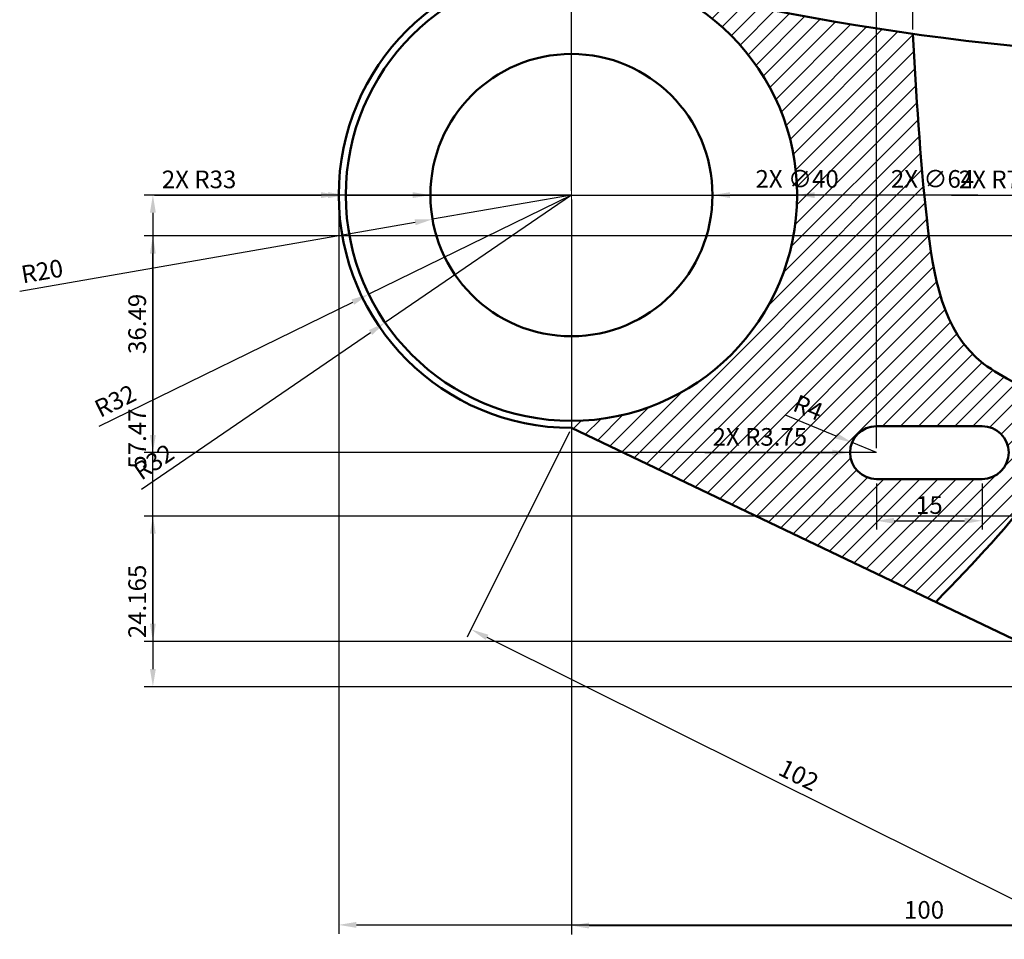
# Model space of a CAD drawing. Units: millimetres. Extents: x 1605 to 2079, y 1280 to 1879.
# Tile 2 of 7: x 1605 to 1745, y 1384 to 1514. Entities that reach past the tile are written whole.
import ezdxf

# ---------------------------------------------------------------- set-up
doc = ezdxf.new("R2010")
doc.units = ezdxf.units.MM
doc.linetypes.add('CENTER2', pattern=[28.574999999999996, 19.05, -3.174999999999999, 3.174999999999999, -3.174999999999999])
for name, color, linetype, lineweight in [('M-CNTR', 1, 'CENTER2', 18), ('M-DIMS', 2, 'Continuous', 25), ('M-HATC', 8, 'Continuous', 18), ('M-OUTL', 7, 'Continuous', 50)]:
    doc.layers.add(name, color=color, linetype=linetype, lineweight=lineweight)
doc.styles.get("Standard").update_dxf_attribs({"font": 'arial.ttf'})
doc.dimstyles.new('ISO-25', dxfattribs={"dimtxt": 2.5, "dimasz": 2.5, "dimexe": 1.25, "dimexo": 0.625, "dimtad": 1, "dimdec": 0, "dimtxsty": 'Standard', "dimcen": 2.5, "dimadec": 0, "dimazin": 0, "dimtfac": 1, "dimtdec": 0, "dimtmove": 0, "dimatfit": 3, "dimfxl": 1, "dimarcsym": 0})

# ---------------------------------------------------------------- blocks, each defined once
blk = doc.blocks.new('*U2')
at = {"layer": 'M-CNTR', "color": 0, "transparency": 16777216}
for p, q in [((0, 6.4), (0, 35.5)), ((-35.5, 0), (-6.399999999999998, 0)), ((6.4, 0), (35.5, 0)), ((0, -35.5), (0, -6.399999999999998))]:
    blk.add_line(p, q, dxfattribs=at)
at = {"layer": 'M-CNTR', "color": 0, "linetype": 'Continuous', "transparency": 16777216}
for p, q in [((0, -3.2), (0, 3.2)), ((-3.2, 0), (3.2, 0))]:
    blk.add_line(p, q, dxfattribs=at)
blk = doc.blocks.new('*D12')
at = {"layer": 'Defpoints', "color": 0, "transparency": 16777216}
for p in [(1650.415855978972, 1488.98060105796), (1916.415855978972, 1488.98060105796), (1916.415855978972, 1385.555788157088)]:
    blk.add_point(p, dxfattribs=at)
at = {"layer": 'M-DIMS', "color": 0, "lineweight": -2, "transparency": 16777216}
for p, q in [((1650.415855978972, 1488.35560105796), (1650.415855978972, 1384.305788157088)), ((1916.415855978972, 1488.35560105796), (1916.415855978972, 1384.305788157088)), ((1652.915855978972, 1385.555788157088), (1913.915855978972, 1385.555788157088))]:
    blk.add_line(p, q, dxfattribs=at)
at = {"layer": 'M-DIMS', "color": 0, "transparency": 16777216}
for points in [[(1652.915855978972, 1385.972454823755), (1652.915855978972, 1385.139121490422), (1650.415855978972, 1385.555788157088)], [(1913.915855978972, 1385.972454823755), (1913.915855978972, 1385.139121490422), (1916.415855978972, 1385.555788157088)]]:
    blk.add_solid(points, dxfattribs=at)
at = {"layer": 'M-DIMS', "color": 0, "transparency": 16777216, "insert": (1783.415855978972, 1387.457220626393), "char_height": 2.5, "attachment_point": 5}
blk.add_mtext('266', dxfattribs=at)
blk = doc.blocks.new('*D14')
at = {"layer": 'Defpoints', "color": 0, "transparency": 16777216}
for p in [(1683.415855978973, 1488.98060105796), (1654.670127227685, 1474.920619601452)]:
    blk.add_point(p, dxfattribs=at)
at = {"layer": 'M-DIMS', "color": 0, "lineweight": -2, "transparency": 16777216}
for p, q in [((1683.415855978973, 1488.98060105796), (1654.670127227685, 1474.920619601452)), ((1616.470490142547, 1456.236585054639), (1652.42436716899, 1473.822183550162))]:
    blk.add_line(p, q, dxfattribs=at)
at = {"layer": 'M-DIMS', "color": 0, "transparency": 16777216}
blk.add_solid([(1652.241294493775, 1474.196476893278), (1652.607439844205, 1473.447890207046), (1654.670127227685, 1474.920619601452)], dxfattribs=at)
at = {"layer": 'M-DIMS', "color": 0, "transparency": 16777216, "insert": (1618.867741976558, 1459.526758746126), "char_height": 2.5, "attachment_point": 5, "rotation": 26.063973519573043}
blk.add_mtext('R32', dxfattribs=at)
blk = doc.blocks.new('*D15')
at = {"layer": 'Defpoints', "color": 0, "transparency": 16777216}
for p in [(1683.415855978971, 1488.98060105796), (1656.997927559478, 1470.92255415298)]:
    blk.add_point(p, dxfattribs=at)
at = {"layer": 'M-DIMS', "color": 0, "lineweight": -2, "transparency": 16777216}
for p, q in [((1683.415855978971, 1488.98060105796), (1656.997927559478, 1470.92255415298)), ((1622.466120198724, 1447.318243204279), (1654.934026901705, 1469.511769238528))]:
    blk.add_line(p, q, dxfattribs=at)
at = {"layer": 'M-DIMS', "color": 0, "transparency": 16777216}
blk.add_solid([(1654.69889608263, 1469.85575268149), (1655.16915772078, 1469.167785795566), (1656.997927559478, 1470.92255415298)], dxfattribs=at)
at = {"layer": 'M-DIMS', "color": 0, "transparency": 16777216, "insert": (1624.363890844126, 1450.919704831629), "char_height": 2.5, "attachment_point": 5, "rotation": 34.354665422321524}
blk.add_mtext('R32', dxfattribs=at)
blk = doc.blocks.new('*D16')
at = {"layer": 'Defpoints', "color": 0, "transparency": 16777216}
for p in [(1683.415855978971, 1488.980601057959), (1663.711259292998, 1485.555857353229)]:
    blk.add_point(p, dxfattribs=at)
at = {"layer": 'M-DIMS', "color": 0, "lineweight": -2, "transparency": 16777216}
for p, q in [((1683.415855978971, 1488.980601057959), (1663.711259292998, 1485.555857353229)), ((1605.180206259197, 1475.382908441698), (1661.248184707251, 1485.127764390138))]:
    blk.add_line(p, q, dxfattribs=at)
at = {"layer": 'M-DIMS', "color": 0, "transparency": 16777216}
blk.add_solid([(1661.176835880069, 1485.538276821096), (1661.319533534433, 1484.71725195918), (1663.711259292998, 1485.555857353229)], dxfattribs=at)
at = {"layer": 'M-DIMS', "color": 0, "transparency": 16777216, "insert": (1608.408931110697, 1477.874012688988), "char_height": 2.5, "attachment_point": 5, "rotation": 9.859759404973948}
blk.add_mtext('R20', dxfattribs=at)
blk = doc.blocks.new('*D24')
at = {"layer": 'Defpoints', "color": 0, "transparency": 16777216}
for p in [(1683.415855978972, 1455.980601057961), (1774.34023088235, 1410.708833274267), (1760.124148162526, 1382.157077993787)]:
    blk.add_point(p, dxfattribs=at)
at = {"layer": 'M-DIMS', "color": 0, "lineweight": -2, "transparency": 16777216}
for p, q in [((1683.1372852421, 1455.421116165798), (1668.642631785403, 1426.309875993155)), ((1671.437712827799, 1426.314562829992), (1757.886208593874, 1383.271360941276)), ((1774.061660145477, 1410.149348382104), (1759.567006688781, 1381.038108209462))]:
    blk.add_line(p, q, dxfattribs=at)
at = {"layer": 'M-DIMS', "color": 0, "transparency": 16777216}
for points in [[(1671.623426652381, 1426.6875527581), (1671.251999003217, 1425.941572901883), (1669.199773259148, 1427.42884577748)], [(1758.071922418456, 1383.644350869385), (1757.700494769293, 1382.898371013168), (1760.124148162526, 1382.157077993787)]]:
    blk.add_solid(points, dxfattribs=at)
at = {"layer": 'M-DIMS', "color": 0, "transparency": 16777216, "insert": (1715.509454221376, 1406.495078269704), "char_height": 2.5, "attachment_point": 5, "rotation": 333.5310232172807}
blk.add_mtext('102', dxfattribs=at)
blk = doc.blocks.new('*D26')
at = {"layer": 'Defpoints', "color": 0, "transparency": 16777216}
for p in [(1726.66629323774, 1448.737829432783), (1741.66629323774, 1448.737829432783), (1741.66629323774, 1442.830488730683)]:
    blk.add_point(p, dxfattribs=at)
at = {"layer": 'M-DIMS', "color": 0, "lineweight": -2, "transparency": 16777216}
for p, q in [((1726.66629323774, 1448.112829432783), (1726.66629323774, 1441.580488730683)), ((1741.66629323774, 1448.112829432783), (1741.66629323774, 1441.580488730683)), ((1729.16629323774, 1442.830488730683), (1739.16629323774, 1442.830488730683))]:
    blk.add_line(p, q, dxfattribs=at)
at = {"layer": 'M-DIMS', "color": 0, "transparency": 16777216}
for points in [[(1729.16629323774, 1443.24715539735), (1729.16629323774, 1442.413822064016), (1726.66629323774, 1442.830488730683)], [(1739.16629323774, 1443.24715539735), (1739.16629323774, 1442.413822064016), (1741.66629323774, 1442.830488730683)]]:
    blk.add_solid(points, dxfattribs=at)
at = {"layer": 'M-DIMS', "color": 0, "transparency": 16777216, "insert": (1734.16629323774, 1444.731921199987), "char_height": 2.5, "attachment_point": 5}
blk.add_mtext('15', dxfattribs=at)
blk = doc.blocks.new('*D27')
at = {"layer": 'Defpoints', "color": 0, "transparency": 16777216}
for p in [(1723.201111272499, 1453.921361416299), (1726.666293237741, 1452.487829432783)]:
    blk.add_point(p, dxfattribs=at)
at = {"layer": 'M-DIMS', "color": 0, "lineweight": -2, "transparency": 16777216}
for p, q in [((1713.710073993439, 1457.84776575314), (1720.890989962337, 1454.877049405309)), ((1726.666293237741, 1452.487829432783), (1723.201111272499, 1453.921361416299))]:
    blk.add_line(p, q, dxfattribs=at)
at = {"layer": 'M-DIMS', "color": 0, "transparency": 16777216}
blk.add_solid([(1721.050271293839, 1455.262069623669), (1720.731708630835, 1454.492029186949), (1723.201111272499, 1453.921361416299)], dxfattribs=at)
at = {"layer": 'M-DIMS', "color": 0, "transparency": 16777216, "insert": (1716.862237314565, 1458.57284255635), "char_height": 2.5, "attachment_point": 5, "rotation": 337.52531510139886}
blk.add_mtext('R4', dxfattribs=at)
blk = doc.blocks.new('*D41')
at = {"layer": 'Defpoints', "color": 0, "transparency": 16777216}
for p in [(1763.415856000001, 1443.479022), (1624.065856000002, 1419.31445), (1783.415856000001, 1419.31445)]:
    blk.add_point(p, dxfattribs=at)
at = {"layer": 'M-DIMS', "color": 0, "lineweight": -2, "transparency": 16777216}
for p, q in [((1762.790856000001, 1443.479022), (1622.815856000002, 1443.479022)), ((1624.065856000002, 1440.979022), (1624.065856000002, 1421.81445)), ((1782.790856000001, 1419.31445), (1622.815856000002, 1419.31445))]:
    blk.add_line(p, q, dxfattribs=at)
at = {"layer": 'M-DIMS', "color": 0, "transparency": 16777216}
for points in [[(1623.649189333335, 1440.979022), (1624.482522666668, 1440.979022), (1624.065856000002, 1443.479022)], [(1623.649189333335, 1421.81445), (1624.482522666668, 1421.81445), (1624.065856000002, 1419.31445)]]:
    blk.add_solid(points, dxfattribs=at)
at = {"layer": 'M-DIMS', "color": 0, "transparency": 16777216, "insert": (1622.164423530697, 1431.396736), "char_height": 2.5, "attachment_point": 5, "rotation": 90}
blk.add_mtext('24.165', dxfattribs=at)
blk = doc.blocks.new('*D42')
at = {"layer": 'Defpoints', "color": 0, "transparency": 16777216}
for p in [(1683.415856, 1488.980601), (1783.415856, 1443.479022), (1783.415856, 1385.46445)]:
    blk.add_point(p, dxfattribs=at)
at = {"layer": 'M-DIMS', "color": 0, "lineweight": -2, "transparency": 16777216}
for p, q in [((1683.415856, 1488.355601), (1683.415856, 1384.21445)), ((1783.415856, 1442.854022), (1783.415856, 1384.21445)), ((1685.915856, 1385.46445), (1780.915856, 1385.46445))]:
    blk.add_line(p, q, dxfattribs=at)
at = {"layer": 'M-DIMS', "color": 0, "transparency": 16777216}
for points in [[(1685.915856, 1385.881116666667), (1685.915856, 1385.047783333333), (1683.415856, 1385.46445)], [(1780.915856, 1385.881116666667), (1780.915856, 1385.047783333333), (1783.415856, 1385.46445)]]:
    blk.add_solid(points, dxfattribs=at)
at = {"layer": 'M-DIMS', "color": 0, "transparency": 16777216, "insert": (1733.415856, 1387.365882469304), "char_height": 2.5, "attachment_point": 5}
blk.add_mtext('100', dxfattribs=at)
blk = doc.blocks.new('*D45')
at = {"layer": 'Defpoints', "color": 0, "transparency": 16777216}
for p in [(1763.415856, 1548.330601), (1683.415856, 1488.980601), (1763.415856, 1488.980601)]:
    blk.add_point(p, dxfattribs=at)
at = {"layer": 'M-DIMS', "color": 0, "lineweight": -2, "transparency": 16777216}
for p, q in [((1683.415856, 1489.605601), (1683.415856, 1549.580601)), ((1685.915856, 1548.330601), (1760.915856, 1548.330601)), ((1763.415856, 1489.605601), (1763.415856, 1549.580601))]:
    blk.add_line(p, q, dxfattribs=at)
at = {"layer": 'M-DIMS', "color": 0, "transparency": 16777216}
for points in [[(1685.915856, 1548.747267666666), (1685.915856, 1547.913934333333), (1683.415856, 1548.330601)], [(1760.915856, 1548.747267666666), (1760.915856, 1547.913934333333), (1763.415856, 1548.330601)]]:
    blk.add_solid(points, dxfattribs=at)
at = {"layer": 'M-DIMS', "color": 0, "transparency": 16777216, "insert": (1723.415856, 1550.232033469304), "char_height": 2.5, "attachment_point": 5}
blk.add_mtext('80', dxfattribs=at)
blk = doc.blocks.new('*D47')
at = {"layer": 'Defpoints', "color": 0, "transparency": 16777216}
for p in [(1726.666293, 1548.330601), (1683.415856, 1488.980601), (1726.666293, 1452.487829)]:
    blk.add_point(p, dxfattribs=at)
at = {"layer": 'M-DIMS', "color": 0, "lineweight": -2, "transparency": 16777216}
for p, q in [((1683.415856, 1489.605601), (1683.415856, 1549.580601)), ((1685.915856, 1548.330601), (1724.166293, 1548.330601)), ((1726.666293, 1453.112829), (1726.666293, 1549.580601))]:
    blk.add_line(p, q, dxfattribs=at)
at = {"layer": 'M-DIMS', "color": 0, "transparency": 16777216}
for points in [[(1685.915856, 1548.747267666666), (1685.915856, 1547.913934333333), (1683.415856, 1548.330601)], [(1724.166293, 1548.747267666666), (1724.166293, 1547.913934333333), (1726.666293, 1548.330601)]]:
    blk.add_solid(points, dxfattribs=at)
at = {"layer": 'M-DIMS', "color": 0, "transparency": 16777216, "insert": (1705.0410745, 1550.232886129604), "char_height": 2.5, "attachment_point": 5}
blk.add_mtext('43.25', dxfattribs=at)
blk = doc.blocks.new('*D48')
at = {"layer": 'Defpoints', "color": 0, "transparency": 16777216}
for p in [(1683.415856000001, 1488.980601), (1624.065856000002, 1452.487829), (1726.666293000001, 1452.487829)]:
    blk.add_point(p, dxfattribs=at)
at = {"layer": 'M-DIMS', "color": 0, "lineweight": -2, "transparency": 16777216}
for p, q in [((1682.790856000001, 1488.980601), (1622.815856000002, 1488.980601)), ((1624.065856000002, 1486.480601), (1624.065856000002, 1454.987829)), ((1726.041293000001, 1452.487829), (1622.815856000002, 1452.487829))]:
    blk.add_line(p, q, dxfattribs=at)
at = {"layer": 'M-DIMS', "color": 0, "transparency": 16777216}
for points in [[(1623.649189333335, 1486.480601), (1624.482522666668, 1486.480601), (1624.065856000002, 1488.980601)], [(1623.649189333335, 1454.987829), (1624.482522666668, 1454.987829), (1624.065856000002, 1452.487829)]]:
    blk.add_solid(points, dxfattribs=at)
at = {"layer": 'M-DIMS', "color": 0, "transparency": 16777216, "insert": (1622.163570870397, 1470.734215), "char_height": 2.5, "attachment_point": 5, "rotation": 90}
blk.add_mtext('36.49', dxfattribs=at)
blk = doc.blocks.new('*D49')
at = {"layer": 'Defpoints', "color": 0, "transparency": 16777216}
for p in [(1731.842463, 1548.330601), (1731.842463, 1511.839336), (1683.415856, 1488.980601)]:
    blk.add_point(p, dxfattribs=at)
at = {"layer": 'M-DIMS', "color": 0, "lineweight": -2, "transparency": 16777216}
for p, q in [((1683.415856, 1489.605601), (1683.415856, 1549.580601)), ((1685.915856, 1548.330601), (1729.342463, 1548.330601)), ((1731.842463, 1512.464336), (1731.842463, 1549.580601))]:
    blk.add_line(p, q, dxfattribs=at)
at = {"layer": 'M-DIMS', "color": 0, "transparency": 16777216}
for points in [[(1685.915856, 1548.747267666666), (1685.915856, 1547.913934333333), (1683.415856, 1548.330601)], [(1729.342463, 1548.747267666666), (1729.342463, 1547.913934333333), (1731.842463, 1548.330601)]]:
    blk.add_solid(points, dxfattribs=at)
at = {"layer": 'M-DIMS', "color": 0, "transparency": 16777216, "insert": (1707.6291595, 1550.232886129604), "char_height": 2.5, "attachment_point": 5}
blk.add_mtext('48.43', dxfattribs=at)
blk = doc.blocks.new('*D51')
at = {"layer": 'Defpoints', "color": 0, "transparency": 16777216}
for p in [(1624.065856000002, 1483.204576), (1984.756367000001, 1483.204576), (1947.568769000001, 1425.734399)]:
    blk.add_point(p, dxfattribs=at)
at = {"layer": 'M-DIMS', "color": 0, "lineweight": -2, "transparency": 16777216}
for p, q in [((1984.131367000001, 1483.204576), (1622.815856000002, 1483.204576)), ((1624.065856000002, 1428.234399), (1624.065856000002, 1480.704576000001)), ((1946.943769000001, 1425.734399), (1622.815856000002, 1425.734399))]:
    blk.add_line(p, q, dxfattribs=at)
at = {"layer": 'M-DIMS', "color": 0, "transparency": 16777216}
for points in [[(1623.649189333335, 1480.704576000001), (1624.482522666668, 1480.704576000001), (1624.065856000002, 1483.204576)], [(1623.649189333335, 1428.234399), (1624.482522666668, 1428.234399), (1624.065856000002, 1425.734399)]]:
    blk.add_solid(points, dxfattribs=at)
at = {"layer": 'M-DIMS', "color": 0, "transparency": 16777216, "insert": (1622.169539492498, 1454.4694875), "char_height": 2.5, "attachment_point": 5, "rotation": 90}
blk.add_mtext('57.47', dxfattribs=at)
blk = doc.blocks.new('*D61')
at = {"layer": 'Defpoints', "color": 0, "transparency": 16777216}
for p in [(1650.415856, 1488.981), (1683.415856, 1488.980601)]:
    blk.add_point(p, dxfattribs=at)
at = {"layer": 'M-DIMS', "color": 0, "lineweight": -2, "transparency": 16777216}
for p, q in [((1624.296790517598, 1488.981315803246), (1647.915856000183, 1488.981030227273)), ((1683.415856, 1488.980601), (1650.415856, 1488.981))]:
    blk.add_line(p, q, dxfattribs=at)
at = {"layer": 'M-DIMS', "color": 0, "transparency": 16777216}
blk.add_solid([(1647.915861038061, 1489.397696893909), (1647.915850962304, 1488.564363560636), (1650.415856, 1488.981)], dxfattribs=at)
at = {"layer": 'M-DIMS', "color": 0, "transparency": 16777216, "insert": (1630.615879001804, 1490.883524529465), "char_height": 2.5, "attachment_point": 5, "rotation": 359.9993072419386}
blk.add_mtext('2X R33', dxfattribs=at)
blk = doc.blocks.new('*D62')
at = {"layer": 'Defpoints', "color": 0, "transparency": 16777216}
for p in [(1651.415856, 1488.980202), (1715.415856, 1488.981)]:
    blk.add_point(p, dxfattribs=at)
at = {"layer": 'M-DIMS', "color": 0, "lineweight": -2, "transparency": 16777216}
for p, q in [((1648.915856000195, 1488.980170828124), (1646.415856000389, 1488.980139656249)), ((1651.415856, 1488.980202), (1715.415856, 1488.981)), ((1741.027008794735, 1488.981319339061), (1717.915855999805, 1488.981031171875))]:
    blk.add_line(p, q, dxfattribs=at)
at = {"layer": 'M-DIMS', "color": 0, "transparency": 16777216}
for points in [[(1648.915850804882, 1489.396837494759), (1648.915861195507, 1488.56350416149), (1651.415856, 1488.980202)], [(1717.915850804493, 1489.397697838509), (1717.915861195118, 1488.564364505241), (1715.415856, 1488.981)]]:
    blk.add_solid(points, dxfattribs=at)
at = {"layer": 'M-DIMS', "color": 0, "transparency": 16777216, "insert": (1734.61583141823, 1490.952590013762), "char_height": 2.5, "attachment_point": 5, "rotation": 0.0007144067509826848}
blk.add_mtext('2X ∅64', dxfattribs=at)
blk = doc.blocks.new('*D63')
at = {"layer": 'Defpoints', "color": 0, "transparency": 16777216}
for p in [(1663.415856000001, 1488.980202), (1703.415856, 1488.981)]:
    blk.add_point(p, dxfattribs=at)
at = {"layer": 'M-DIMS', "color": 0, "lineweight": -2, "transparency": 16777216}
for p, q in [((1660.915856000498, 1488.980152125), (1658.415856000996, 1488.98010225)), ((1663.415856000001, 1488.980202), (1703.415856, 1488.981)), ((1721.827861453362, 1488.981367319509), (1705.915855999502, 1488.981049875))]:
    blk.add_line(p, q, dxfattribs=at)
at = {"layer": 'M-DIMS', "color": 0, "transparency": 16777216}
for points in [[(1660.915847687998, 1489.396818791584), (1660.915864312998, 1488.563485458416), (1663.415856000001, 1488.980202)], [(1705.915847687002, 1489.397716541584), (1705.915864312003, 1488.564383208416), (1703.415856, 1488.981)]]:
    blk.add_solid(points, dxfattribs=at)
at = {"layer": 'M-DIMS', "color": 0, "transparency": 16777216, "insert": (1715.415816669167, 1490.952590013523), "char_height": 2.5, "attachment_point": 5, "rotation": 0.001143050800851883}
blk.add_mtext('2X ∅40', dxfattribs=at)
blk = doc.blocks.new('*D68')
at = {"layer": 'Defpoints', "color": 0, "transparency": 16777216}
for p in [(1755.915856, 1488.981), (1763.415855999999, 1488.980601)]:
    blk.add_point(p, dxfattribs=at)
at = {"layer": 'M-DIMS', "color": 0, "lineweight": -2, "transparency": 16777216}
for p, q in [((1737.288639109579, 1488.981990967938), (1753.415856003538, 1488.981133)), ((1763.415855999999, 1488.980601), (1755.915856, 1488.981))]:
    blk.add_line(p, q, dxfattribs=at)
at = {"layer": 'M-DIMS', "color": 0, "transparency": 16777216}
blk.add_solid([(1753.415878170204, 1489.397799666077), (1753.415833836871, 1488.564466333922), (1755.915856, 1488.981)], dxfattribs=at)
at = {"layer": 'M-DIMS', "color": 0, "transparency": 16777216, "insert": (1744.102348714535, 1490.883060950582), "char_height": 2.5, "attachment_point": 5, "rotation": 359.99695186453266}
blk.add_mtext('2X R7.5', dxfattribs=at)
blk = doc.blocks.new('*D69')
at = {"layer": 'Defpoints', "color": 0, "transparency": 16777216}
for p in [(1722.916293, 1452.488), (1726.666293, 1452.487829)]:
    blk.add_point(p, dxfattribs=at)
at = {"layer": 'M-DIMS', "color": 0, "lineweight": -2, "transparency": 16777216}
for p, q in [((1702.346715940895, 1452.488937972713), (1720.416293002599, 1452.488114)), ((1726.666293, 1452.487829), (1722.916293, 1452.488))]:
    blk.add_line(p, q, dxfattribs=at)
at = {"layer": 'M-DIMS', "color": 0, "transparency": 16777216}
blk.add_solid([(1720.416312002599, 1452.904780666233), (1720.416274002599, 1452.071447333766), (1722.916293, 1452.488)], dxfattribs=at)
at = {"layer": 'M-DIMS', "color": 0, "transparency": 16777216, "insert": (1710.131591217248, 1454.390868113983), "char_height": 2.5, "attachment_point": 5, "rotation": 359.9973873124574}
blk.add_mtext('2X R3.75', dxfattribs=at)

msp = doc.modelspace()

# ---------------------------------------------------------------- hatches: boundary and pattern name
at = {"layer": 'M-HATC'}
h = msp.add_hatch(dxfattribs=at)
h.set_pattern_fill('ANSI31', color=256, scale=0.5700000000000001)
h.set_pattern_definition([(45, (0, 0), (-1.279686497252354, 1.279686497252354), [])])
edge = h.paths.add_edge_path()
edge.add_spline(control_points=[(1735.07459974606, 1431.314795075923), (1745.983278041014, 1442.572726331581), (1760.24984788448, 1457.296055612093), (1736.483989804082, 1465.949384402775), (1733.184296285201, 1487.573131299177), (1732.318614147286, 1503.228440483471), (1731.842462696298, 1511.83933570387)], knot_values=[0, 0, 0, 0, 32.3106591245444, 42.25647348148218, 64.0151754338639, 90.61240603446909, 90.61240603446909, 90.61240603446909, 90.61240603446909], degree=3, periodic=0)
edge.add_arc((1783.415855978972, 1878.806874192082), 370.5738647001252, 256.0328658121666, 262.00008128327465, ccw=False)
edge.add_arc((1683.415855978972, 1488.98060105796), 32, 0, 70.73817384477002, ccw=False)
edge.add_arc((1683.415855978972, 1488.98060105796), 32, -90, 0, ccw=False)
edge.add_line((1683.415855978972, 1456.98060105796), (1683.415855978972, 1455.98060105796))
edge.add_line((1683.415855978972, 1455.98060105796), (1735.07459974606, 1431.314795075923))
h.paths.add_polyline_path([(1726.66629323774, 1456.237829432783), (1741.66629323774, 1456.237829432783, -1), (1741.66629323774, 1448.737829432783), (1726.66629323774, 1448.737829432783, -1)], flags=16)
h.paths.add_polyline_path([(1731.47870797171, 1442.133012605171), (1736.613428299132, 1442.133012605171), (1736.613428299132, 1447.284786138595), (1731.47870797171, 1447.284786138595)], flags=24)
h.paths.add_polyline_path([(1713.173444990596, 1457.268825178529), (1718.453947385105, 1455.084302360538), (1720.423342620304, 1459.844791090414), (1715.142840225795, 1462.029313908404)], flags=24)

# ---------------------------------------------------------------- linework, layer by layer
at = {"layer": 'M-OUTL'}
for p, q in [((1726.66629323774, 1456.237829432783), (1741.66629323774, 1456.237829432783)), ((1683.415855978972, 1455.98060105796), (1779.107066766559, 1410.29035256654)), ((1741.66629323774, 1448.737829432783), (1726.66629323774, 1448.737829432783))]:
    msp.add_line(p, q, dxfattribs=at)
for radius in [32, 20]:
    msp.add_circle((1683.415855978972, 1488.98060105796), radius, dxfattribs=at)
for centre, radius, start, end in [((1683.415855978972, 1488.98060105796), 33, 90, 270), ((1783.415855978972, 1878.806874192082), 370.5738647001254, 254.3445556403036, 285.6554443596963), ((1726.66629323774, 1452.487829432782), 3.75, 90, 270), ((1741.66629323774, 1452.487829432782), 3.75, 270, 90)]:
    msp.add_arc(centre, radius, start, end, dxfattribs=at)
msp.add_open_spline([(1731.842462696298, 1511.83933570387), (1732.318614147286, 1503.228440483471), (1733.184296285201, 1487.573131299177), (1736.483989804081, 1465.949384402775), (1760.24984788448, 1457.296055612093), (1745.983278041014, 1442.572726331581), (1735.07459974606, 1431.314795075923)], degree=3, knots=[0, 0, 0, 0, 26.59723060060519, 48.35593255298691, 58.30174690992469, 90.61240603446909, 90.61240603446909, 90.61240603446909, 90.61240603446909], dxfattribs=at)

# ---------------------------------------------------------------- block references
at = {"layer": 'M-CNTR'}
msp.add_blockref('*U2', (1683.415855978972, 1488.98060105796), dxfattribs=at)

# ---------------------------------------------------------------- dimensions: what is measured, and where the dimension line sits
at = {"layer": 'M-DIMS'}
for base, p1, p2, override, picture, middle in [((1726.666293, 1548.330601), (1683.415856, 1488.980601), (1726.666293, 1452.487829), {"dimdec": 2, "dimlfac": 1, "dimrnd": 0, "dimzin": 0, "dimdsep": 46, "dimlunit": 2}, '*D47', (1705.0410745, 1550.232886129604)), ((1731.842463, 1548.330601), (1683.415856, 1488.980601), (1731.842463, 1511.839336), {"dimdec": 2, "dimlfac": 1, "dimrnd": 0, "dimzin": 0, "dimdsep": 46, "dimlunit": 2}, '*D49', (1707.6291595, 1550.232886129604)), ((1763.415856, 1548.330601), (1683.415856, 1488.980601), (1763.415856, 1488.980601), {"dimdec": 0, "dimlfac": 1, "dimrnd": 0, "dimzin": 0, "dimdsep": 46, "dimlunit": 2}, '*D45', (1723.415856, 1550.232033469304)), ((1916.415855978972, 1385.555788157088), (1650.415855978972, 1488.98060105796), (1916.415855978972, 1488.98060105796), {"dimclrd": 0, "dimclre": 0, "dimclrt": 0}, '*D12', (1783.415855978972, 1387.457220626393)), ((1783.415856, 1385.46445), (1683.415856, 1488.980601), (1783.415856, 1443.479022), {"dimdec": 0, "dimlfac": 1, "dimrnd": 0, "dimzin": 0, "dimdsep": 46, "dimlunit": 2}, '*D42', (1733.415856, 1387.365882469304)), ((1741.66629323774, 1442.830488730683), (1726.66629323774, 1448.737829432783), (1741.66629323774, 1448.737829432783), {"dimclrd": 0, "dimclre": 0, "dimclrt": 0}, '*D26', (1734.16629323774, 1444.731921199987))]:
    dim = msp.add_linear_dim(base=base, p1=p1, p2=p2, dimstyle='ISO-25', override=override, dxfattribs=at)
    dim.commit()
    dim.dimension.update_dxf_attribs({"geometry": picture, "text_midpoint": middle})
dim = msp.add_radius_dim(center=(1683.415856, 1488.980601), mpoint=(1650.415856, 1488.981), text='2X <>', dimstyle='ISO-25', override={"dimdec": 0, "dimlfac": 1, "dimrnd": 0, "dimzin": 0, "dimdsep": 46, "dimlunit": 2}, dxfattribs=at)
dim.commit()
dim.dimension.update_dxf_attribs({"geometry": '*D61', "text_midpoint": (1630.615856001448, 1488.9812394), "dimtype": 164})
for p1, p2, picture, middle in [((1651.415856, 1488.980202), (1715.415856, 1488.981), '*D62', (1734.615855998508, 1488.9812394)), ((1663.415856000001, 1488.980202), (1703.415856, 1488.981), '*D63', (1715.415855997612, 1488.9812394))]:
    dim = msp.add_diameter_dim_2p(p1=p1, p2=p2, text='2X <>', dimstyle='ISO-25', override={"dimdec": 0, "dimlfac": 1, "dimrnd": 0, "dimzin": 0, "dimdsep": 46, "dimlunit": 2}, dxfattribs=at)
    dim.commit()
    dim.dimension.update_dxf_attribs({"geometry": picture, "text_midpoint": middle, "dimtype": 163})
for center, mpoint, override, picture, middle in [((1763.415855999999, 1488.980601), (1755.915856, 1488.981), {"dimdec": 1, "dimlfac": 1, "dimrnd": 0, "dimzin": 0, "dimdsep": 46, "dimlunit": 2}, '*D68', (1744.102348714535, 1490.883060950582)), ((1726.666293, 1452.487829), (1722.916293, 1452.488), {"dimdec": 2, "dimlfac": 1, "dimrnd": 0, "dimzin": 0, "dimdsep": 46, "dimlunit": 2}, '*D69', (1710.131591217248, 1454.390868113983))]:
    dim = msp.add_radius_dim(center=center, mpoint=mpoint, text='2X <>', dimstyle='ISO-25', override=override, dxfattribs=at)
    dim.commit()
    dim.dimension.update_dxf_attribs({"geometry": picture, "text_midpoint": middle})
for center, mpoint, picture, middle in [((1683.415855978971, 1488.980601057959), (1663.711259292998, 1485.555857353229), '*D16', (1608.734527054658, 1476.000664692325)), ((1683.415855978973, 1488.98060105796), (1654.670127227685, 1474.920619601452), '*D14', (1619.703557403034, 1457.817928360401)), ((1683.415855978971, 1488.98060105796), (1656.997927559478, 1470.92255415298), '*D15', (1625.437376909658, 1449.349253819525))]:
    dim = msp.add_radius_dim(center=center, mpoint=mpoint, dimstyle='ISO-25', override={"dimclrd": 0, "dimclre": 0, "dimclrt": 0}, dxfattribs=at)
    dim.commit()
    dim.dimension.update_dxf_attribs({"geometry": picture, "text_midpoint": middle, "dimtype": 164})
for base, p1, p2, override, picture, middle in [((1624.065856000002, 1452.487829), (1683.415856, 1488.980601), (1726.666293, 1452.487829), {"dimdec": 2, "dimlfac": 1, "dimrnd": 0, "dimzin": 0, "dimdsep": 46, "dimlunit": 2}, '*D48', (1622.163570870397, 1470.734215)), ((1624.065856000002, 1483.204576), (1947.568769, 1425.734399), (1984.756367, 1483.204576), {"dimdec": 2, "dimlfac": 1, "dimrnd": 0, "dimzin": 0, "dimdsep": 46, "dimlunit": 2}, '*D51', (1622.169539492498, 1454.4694875)), ((1624.065856000002, 1419.31445), (1763.415856, 1443.479022), (1783.415856, 1419.31445), {"dimdec": 3, "dimlfac": 1, "dimrnd": 0, "dimzin": 0, "dimdsep": 46, "dimlunit": 2}, '*D41', (1622.164423530697, 1431.396736))]:
    dim = msp.add_linear_dim(base=base, p1=p1, p2=p2, angle=90, dimstyle='ISO-25', override=override, dxfattribs=at)
    dim.commit()
    dim.dimension.update_dxf_attribs({"geometry": picture, "text_midpoint": middle})
dim = msp.add_radius_dim(center=(1726.666293237741, 1452.487829432783), mpoint=(1723.201111272499, 1453.921361416299), dimstyle='ISO-25', override={"dimclrd": 0, "dimclre": 0, "dimclrt": 0}, dxfattribs=at)
dim.commit()
dim.dimension.update_dxf_attribs({"geometry": '*D27', "text_midpoint": (1716.862237314565, 1458.57284255635)})
dim = msp.add_aligned_dim(p1=(1683.415855978972, 1455.98060105796), p2=(1774.34023088235, 1410.708833274267), distance=-31.895136580571247, dimstyle='ISO-25', override={"dimclrd": 0, "dimclre": 0, "dimclrt": 0}, dxfattribs=at)
dim.commit()
dim.dimension.update_dxf_attribs({"geometry": '*D24', "text_midpoint": (1715.509454221376, 1406.495078269704)})

doc.saveas('drawing.dxf')
